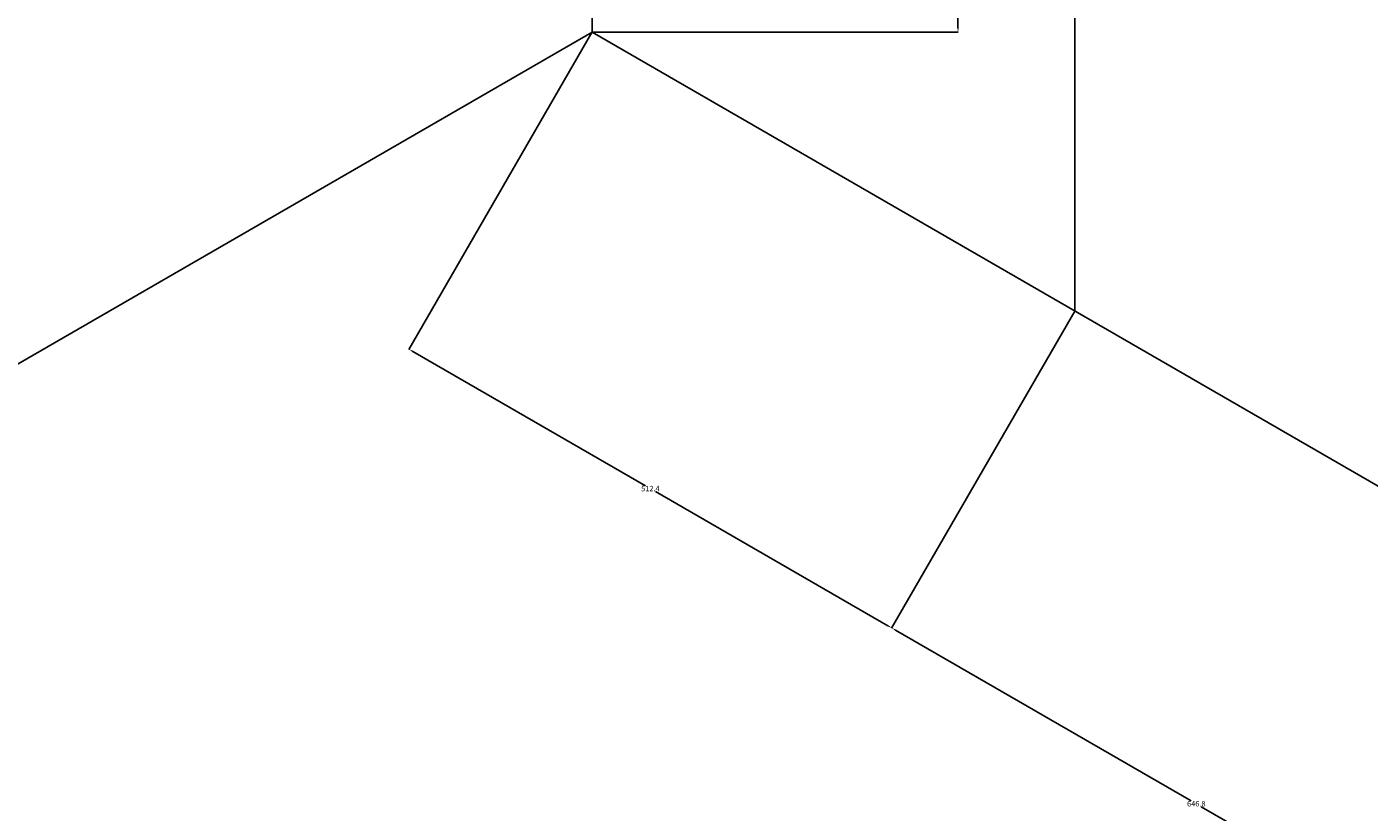
# Model space of a CAD drawing. Units: metres. Extents: x -2391 to 4922, y -635 to 4845.
# Tile 22 of 37: x 31 to 1265, y 1408 to 2130. Entities that reach past the tile are written whole.
import ezdxf

# ---------------------------------------------------------------- set-up
doc = ezdxf.new("R2010")
doc.units = ezdxf.units.M
doc.header["$MEASUREMENT"] = 0
doc.layers.add('A-ANNO-DIMS', color=2, linetype='Continuous', lineweight=18)
doc.layers.add('A-FLOR-FIXT', color=3, linetype='Continuous', lineweight=25)
doc.styles.get("Standard").update_dxf_attribs({"font": 'arial.ttf'})
doc.dimstyles.get("Standard").update_dxf_attribs({"dimtxt": 5, "dimasz": 4, "dimexe": 0.18, "dimexo": 0.0625, "dimgap": 0.09, "dimtad": 0, "dimtih": 1, "dimtoh": 1, "dimdec": 0, "dimzin": 0, "dimdsep": 46, "dimtxsty": 'Standard', "dimcen": 0.09, "dimadec": 0, "dimazin": 0, "dimtfac": 1, "dimtdec": 0, "dimtofl": 0, "dimtmove": 0, "dimatfit": 3, "dimfxl": 1, "dimtolj": 1, "dimtzin": 0, "dimarcsym": 0})

# ---------------------------------------------------------------- blocks, each defined once
blk = doc.blocks.new('*D8')
at = {"layer": 'A-ANNO-DIMS', "color": 0, "lineweight": -2, "transparency": 16777216}
for p, q in [((-2047.3, 3005.2), (-2047.3, -631.4)), ((4577.8, 2350.2), (4577.8, -631.4)), ((-2043.3, -631.2), (1257.6, -631.2)), ((4573.8, -631.2), (1272.8, -631.2))]:
    blk.add_line(p, q, dxfattribs=at)
at = {"layer": 'A-ANNO-DIMS', "color": 0, "transparency": 16777216}
for points in [[(-2043.3, -630.6), (-2043.3, -631.9), (-2047.3, -631.2)], [(4573.8, -630.6), (4573.8, -631.9), (4577.8, -631.2)]]:
    blk.add_solid(points, dxfattribs=at)
at = {"layer": 'Defpoints', "color": 0, "transparency": 16777216}
for p in [(-2047.3, 3005.3), (4577.8, 2350.3), (4577.8, -631.2)]:
    blk.add_point(p, dxfattribs=at)
at = {"layer": 'A-ANNO-DIMS', "color": 0, "transparency": 16777216, "insert": (1265.2, -631.2), "char_height": 5, "attachment_point": 5}
blk.add_mtext('\\A1;6625', dxfattribs=at)
blk = doc.blocks.new('*D10')
at = {"layer": 'A-ANNO-DIMS', "color": 0, "lineweight": -2, "transparency": 16777216}
for p, q in [((550.7, 4505.3), (-2384, 4505.3)), ((-2383.8, 4501.3), (-2383.8, 2107.9)), ((-2383.8, -290.7), (-2383.8, 2102.6)), ((-488.6, -294.7), (-2384, -294.7))]:
    blk.add_line(p, q, dxfattribs=at)
at = {"layer": 'A-ANNO-DIMS', "color": 0, "transparency": 16777216}
for points in [[(-2384.5, 4501.3), (-2383.2, 4501.3), (-2383.8, 4505.3)], [(-2384.5, -290.7), (-2383.2, -290.7), (-2383.8, -294.7)]]:
    blk.add_solid(points, dxfattribs=at)
at = {"layer": 'Defpoints', "color": 0, "transparency": 16777216}
for p in [(-2383.8, 4505.3), (550.7, 4505.3), (-488.5, -294.7)]:
    blk.add_point(p, dxfattribs=at)
at = {"layer": 'A-ANNO-DIMS', "color": 0, "transparency": 16777216, "insert": (-2383.8, 2105.3), "char_height": 5, "attachment_point": 5}
blk.add_mtext('\\A1;4800', dxfattribs=at)
blk = doc.blocks.new('*D11')
at = {"layer": 'A-ANNO-DIMS', "color": 0, "lineweight": -2, "transparency": 16777216}
for p, q in [((550.8, 4505.3), (887.4, 4505.3)), ((887.2, 4501.3), (887.2, 3317.9)), ((887.2, 2129.3), (887.2, 3312.6)), ((550.8, 2125.3), (887.4, 2125.3))]:
    blk.add_line(p, q, dxfattribs=at)
at = {"layer": 'A-ANNO-DIMS', "color": 0, "transparency": 16777216}
for points in [[(886.6, 4501.3), (887.9, 4501.3), (887.2, 4505.3)], [(886.6, 2129.3), (887.9, 2129.3), (887.2, 2125.3)]]:
    blk.add_solid(points, dxfattribs=at)
at = {"layer": 'Defpoints', "color": 0, "transparency": 16777216}
for p in [(550.7, 4505.3), (550.7, 2125.3), (887.2, 2125.3)]:
    blk.add_point(p, dxfattribs=at)
at = {"layer": 'A-ANNO-DIMS', "color": 0, "transparency": 16777216, "insert": (887.2, 3315.3), "char_height": 5, "attachment_point": 5}
blk.add_mtext('\\A1;2380', dxfattribs=at)
blk = doc.blocks.new('*D18')
at = {"layer": 'A-ANNO-DIMS', "color": 0, "lineweight": -2, "transparency": 16777216}
for p, q in [((550.7, 2125.2), (382.4, 1833.7)), ((994.5, 1869), (826.2, 1577.5)), ((386, 1831.9), (599.8, 1708.4)), ((822.8, 1579.6), (609, 1703.1))]:
    blk.add_line(p, q, dxfattribs=at)
at = {"layer": 'A-ANNO-DIMS', "color": 0, "transparency": 16777216}
for points in [[(386.3, 1832.4), (385.6, 1831.3), (382.5, 1833.9)], [(823.1, 1580.2), (822.5, 1579.1), (826.3, 1577.6)]]:
    blk.add_solid(points, dxfattribs=at)
at = {"layer": 'Defpoints', "color": 0, "transparency": 16777216}
for p in [(550.7, 2125.3), (994.5, 1869.1), (382.5, 1833.9)]:
    blk.add_point(p, dxfattribs=at)
at = {"layer": 'A-ANNO-DIMS', "color": 0, "transparency": 16777216, "insert": (604.4, 1705.8), "char_height": 5, "attachment_point": 5}
blk.add_mtext('\\A1;512.4', dxfattribs=at)
blk = doc.blocks.new('*D19')
at = {"layer": 'A-ANNO-DIMS', "color": 0, "lineweight": -2, "transparency": 16777216}
for p, q in [((994.5, 1869), (826.2, 1577.5)), ((829.7, 1575.6), (1101.7, 1418.6)), ((1554.6, 1545.6), (1386.3, 1254.1)), ((1382.9, 1256.3), (1110.9, 1413.3))]:
    blk.add_line(p, q, dxfattribs=at)
at = {"layer": 'A-ANNO-DIMS', "color": 0, "transparency": 16777216}
for points in [[(830.1, 1576.2), (829.4, 1575.1), (826.3, 1577.6)], [(1383.2, 1256.8), (1382.6, 1255.7), (1386.4, 1254.3)]]:
    blk.add_solid(points, dxfattribs=at)
at = {"layer": 'Defpoints', "color": 0, "transparency": 16777216}
for p in [(994.5, 1869.1), (826.3, 1577.6), (1554.6, 1545.7)]:
    blk.add_point(p, dxfattribs=at)
at = {"layer": 'A-ANNO-DIMS', "color": 0, "transparency": 16777216, "insert": (1106.3, 1416), "char_height": 5, "attachment_point": 5}
blk.add_mtext('\\A1;646.8', dxfattribs=at)
blk = doc.blocks.new('*D24')
at = {"layer": 'A-ANNO-DIMS', "color": 0, "lineweight": -2, "transparency": 16777216}
for p, q in [((550.8, 2947.9), (887.4, 2947.9)), ((887.2, 2943.9), (887.2, 2539.2)), ((887.2, 2129.3), (887.2, 2534)), ((550.8, 2125.3), (887.4, 2125.3))]:
    blk.add_line(p, q, dxfattribs=at)
at = {"layer": 'A-ANNO-DIMS', "color": 0, "transparency": 16777216}
for points in [[(886.6, 2943.9), (887.9, 2943.9), (887.2, 2947.9)], [(886.6, 2129.3), (887.9, 2129.3), (887.2, 2125.3)]]:
    blk.add_solid(points, dxfattribs=at)
at = {"layer": 'Defpoints', "color": 0, "transparency": 16777216}
for p in [(550.7, 2947.9), (550.7, 2125.3), (887.2, 2125.3)]:
    blk.add_point(p, dxfattribs=at)
at = {"layer": 'A-ANNO-DIMS', "color": 0, "transparency": 16777216, "insert": (887.2, 2536.6), "char_height": 5, "attachment_point": 5}
blk.add_mtext('\\A1;822.6', dxfattribs=at)

msp = doc.modelspace()

# ---------------------------------------------------------------- linework, layer by layer
at = {"layer": 'A-FLOR-FIXT'}
for p, q in [((550.7419, 2947.9199), (550.7419, 2125.2763)), ((994.5103, 2691.71), (994.5103, 1869.0664)), ((550.7419, 2125.2763), (-765.6167, 1365.2763)), ((3148.8181, 625.2763), (550.7419, 2125.2763))]:
    msp.add_line(p, q, dxfattribs=at)

# ---------------------------------------------------------------- dimensions: what is measured, and where the dimension line sits
at = {"layer": 'A-ANNO-DIMS'}
for base, p1, p2, angle, override, picture, middle in [((-2383.8343, 4505.2763), (-488.4886, -294.7237), (550.7419, 4505.2763), 90, {"dimdec": 0, "dimlfac": 1, "dimrnd": 0, "dimzin": 0, "dimdsep": 46, "dimlunit": 2}, '*D10', (-2383.8343, 2105.2763)), ((887.2419, 2125.2763), (550.7419, 4505.2763), (550.7419, 2125.2763), 270, {"dimdec": 0, "dimlfac": 1, "dimrnd": 0, "dimzin": 0, "dimdsep": 46, "dimlunit": 2}, '*D11', (887.2419, 3315.2763)), ((887.2419, 2125.2763), (550.7419, 2947.9199), (550.7419, 2125.2763), 270, {"dimdec": 1, "dimlfac": 1, "dimrnd": 0, "dimzin": 0, "dimdsep": 46, "dimlunit": 2}, '*D24', (887.2419, 2536.5981)), ((382.4919, 1833.8587), (994.5103, 1869.0664), (550.7419, 2125.2763), 150, {"dimdec": 1, "dimlfac": 1, "dimrnd": 0, "dimzin": 0, "dimdsep": 46, "dimlunit": 2}, '*D18', (604.3761, 1705.7538)), ((826.2603, 1577.6489), (1554.6155, 1545.6896), (994.5103, 1869.0664), 150, {"dimdec": 1, "dimlfac": 1, "dimrnd": 0, "dimzin": 0, "dimdsep": 46, "dimlunit": 2}, '*D19', (1106.3129, 1415.9604))]:
    dim = msp.add_linear_dim(base=base, p1=p1, p2=p2, angle=angle, dimstyle='Standard', override=override, dxfattribs=at)
    dim.commit()
    dim.dimension.update_dxf_attribs({"geometry": picture, "text_midpoint": middle})
dim = msp.add_linear_dim(base=(4577.76, -631.2237), p1=(-2047.3343, 3005.2763), p2=(4577.76, 2350.2763), dimstyle='Standard', override={"dimdec": 0, "dimlfac": 1, "dimrnd": 0, "dimzin": 0, "dimdsep": 46, "dimlunit": 2}, dxfattribs=at)
dim.commit()
dim.dimension.update_dxf_attribs({"geometry": '*D8', "text_midpoint": (1265.2128, -631.2237)})

doc.saveas('drawing.dxf')
